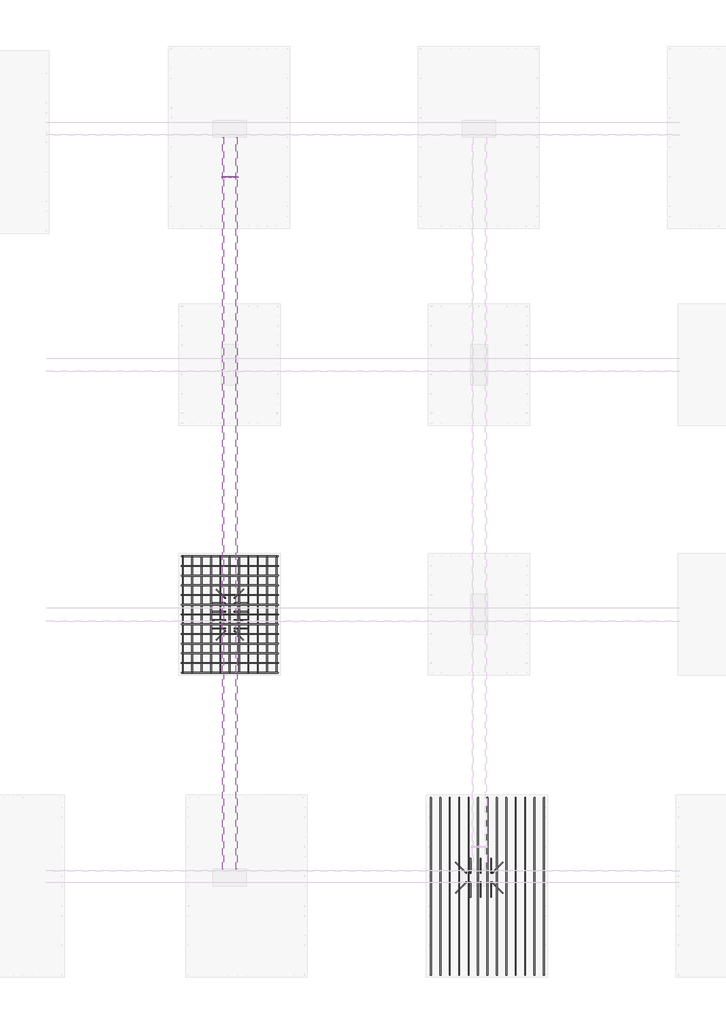
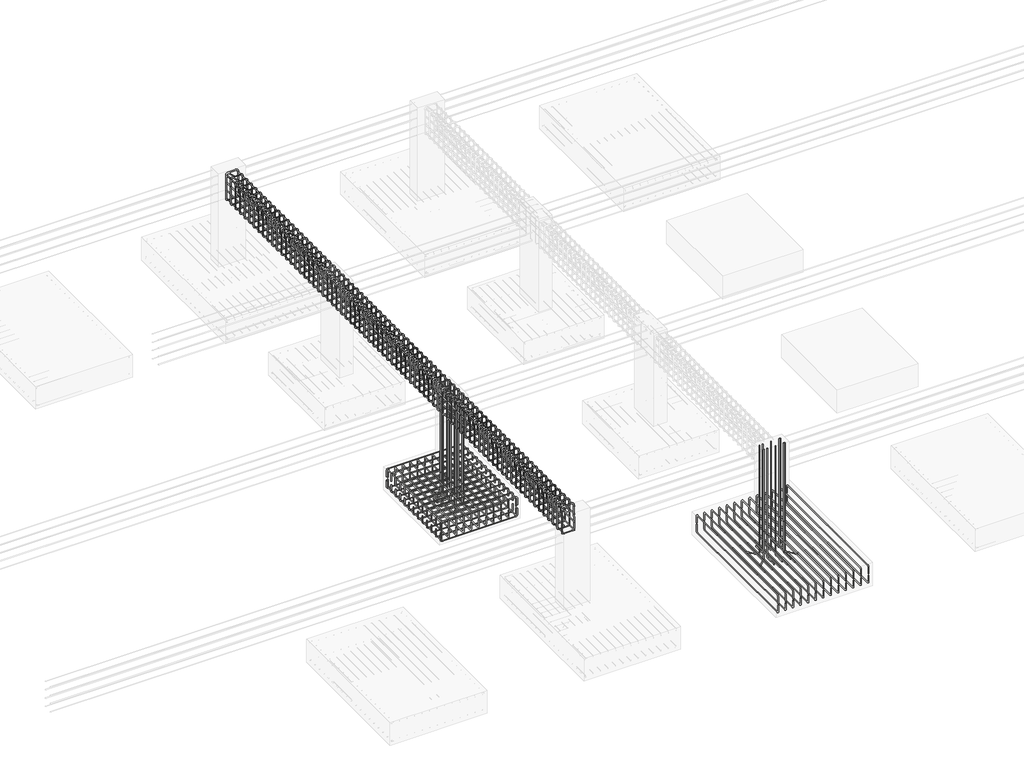
# One storey, part 5 of 16: 21 reinforcing bars.
"""IFC4 building model written with IfcOpenShell, lengths in millimetres."""

from ifc_helpers import new_model, si_unit, point, frame, origin, place, context, project, spatial, polyline, circle_curve, trimmed, segment, composite_curve, source, transform, mapped, element, save
from ifc_brep_helpers import swept_disk

model = new_model("IFC4")

# Units and contexts
model_context = context("Model", 3, world=origin())
ifc_project = project(units=[si_unit("LENGTHUNIT", "METRE", prefix="MILLI")], contexts=[model_context])

# Site, building, storey
site = spatial("IfcSite", under=ifc_project)
building = spatial("IfcBuilding", under=site)
storey = spatial("IfcBuildingStorey", under=building, Elevation=-1828.8)

# Reinforcing bars
placement = place(None, origin())
reinforcing_bar_shape = source(origin(), model_context, "Body", "SolidModel", [
    swept_disk(composite_curve([segment(polyline([(-2445.6525168, -5094.4085501, -2074.8303715), (-2445.6525168, -5094.4085501, -2198.8303715)]), True, "CONTINUOUS"), segment(trimmed(circle_curve(frame((-2445.6525168, -5124.4085501, -2198.8303715), z_axis=(-1.0, 0.0, 0.0), x_axis=(0.0, 30.0, 0.0)), 30.0), [point((-2445.6525168, -5094.4085501, -2198.8303715))], [point((-2445.6525168, -5124.4085501, -2228.8303715))], True, "CARTESIAN"), True, "CONTINUOUS"), segment(polyline([(-2445.6525168, -5124.4085501, -2228.8303715), (-2445.6525168, -7692.4085501, -2228.8303715)]), True, "CONTINUOUS"), segment(trimmed(circle_curve(frame((-2445.6525168, -7692.4085501, -2198.8303715), z_axis=(-1.0, 0.0, 0.0), x_axis=(0.0, 0.0, -30.0)), 30.0), [point((-2445.6525168, -7692.4085501, -2228.8303715))], [point((-2445.6525168, -7722.4085501, -2198.8303715))], True, "CARTESIAN"), True, "CONTINUOUS"), segment(polyline([(-2445.6525168, -7722.4085501, -2198.8303715), (-2445.6525168, -7722.4085501, -2074.8303715)]), True, "CONTINUOUS")], self_intersect=False), 6.0),
])
element("IfcReinforcingBar", 1, at=placement, inside=storey, context=model_context, shape_type="MappedRepresentation", body=[
    mapped(reinforcing_bar_shape, transform((0.0, 0.0, 0.0), x_axis=(1.0, 0.0, 0.0), y_axis=(0.0, 1.0, 0.0), z_axis=(0.0, 0.0, 1.0))),
    mapped(reinforcing_bar_shape, transform((139.7704391, 0.0, 0.0), x_axis=(1.0, 0.0, 0.0), y_axis=(0.0, 1.0, 0.0), z_axis=(0.0, 0.0, 1.0))),
    mapped(reinforcing_bar_shape, transform((279.5408781, 0.0, 0.0), x_axis=(1.0, 0.0, 0.0), y_axis=(0.0, 1.0, 0.0), z_axis=(0.0, 0.0, 1.0))),
    mapped(reinforcing_bar_shape, transform((419.3113172, 0.0, 0.0), x_axis=(1.0, 0.0, 0.0), y_axis=(0.0, 1.0, 0.0), z_axis=(0.0, 0.0, 1.0))),
    mapped(reinforcing_bar_shape, transform((559.0817562, 0.0, 0.0), x_axis=(1.0, 0.0, 0.0), y_axis=(0.0, 1.0, 0.0), z_axis=(0.0, 0.0, 1.0))),
    mapped(reinforcing_bar_shape, transform((698.8521953, 0.0, 0.0), x_axis=(1.0, 0.0, 0.0), y_axis=(0.0, 1.0, 0.0), z_axis=(0.0, 0.0, 1.0))),
    mapped(reinforcing_bar_shape, transform((838.6226343, 0.0, 0.0), x_axis=(1.0, 0.0, 0.0), y_axis=(0.0, 1.0, 0.0), z_axis=(0.0, 0.0, 1.0))),
    mapped(reinforcing_bar_shape, transform((978.3930734, 0.0, 0.0), x_axis=(1.0, 0.0, 0.0), y_axis=(0.0, 1.0, 0.0), z_axis=(0.0, 0.0, 1.0))),
    mapped(reinforcing_bar_shape, transform((1118.1635125, 0.0, 0.0), x_axis=(1.0, 0.0, 0.0), y_axis=(0.0, 1.0, 0.0), z_axis=(0.0, 0.0, 1.0))),
    mapped(reinforcing_bar_shape, transform((1257.9339515, 0.0, 0.0), x_axis=(1.0, 0.0, 0.0), y_axis=(0.0, 1.0, 0.0), z_axis=(0.0, 0.0, 1.0))),
    mapped(reinforcing_bar_shape, transform((1397.7043906, 0.0, 0.0), x_axis=(1.0, 0.0, 0.0), y_axis=(0.0, 1.0, 0.0), z_axis=(0.0, 0.0, 1.0))),
    mapped(reinforcing_bar_shape, transform((1537.4748296, 0.0, 0.0), x_axis=(1.0, 0.0, 0.0), y_axis=(0.0, 1.0, 0.0), z_axis=(0.0, 0.0, 1.0))),
    mapped(reinforcing_bar_shape, transform((1677.2452687, 0.0, 0.0), x_axis=(1.0, 0.0, 0.0), y_axis=(0.0, 1.0, 0.0), z_axis=(0.0, 0.0, 1.0))),
])
reinforcing_bar_2_shape = source(origin(), model_context, "Body", "SolidModel", [
    swept_disk(composite_curve([segment(polyline([(-768.4072481, -5094.4085501, -2038.9453456), (-768.4072481, -5094.4085501, -1914.9453456)]), True, "CONTINUOUS"), segment(trimmed(circle_curve(frame((-768.4072481, -5124.4085501, -1914.9453456), z_axis=(1.0, 0.0, 0.0), x_axis=(0.0, 30.0, 0.0)), 30.0), [point((-768.4072481, -5094.4085501, -1914.9453456))], [point((-768.4072481, -5124.4085501, -1884.9453456))], True, "CARTESIAN"), True, "CONTINUOUS"), segment(polyline([(-768.4072481, -5124.4085501, -1884.9453456), (-768.4072481, -7692.4085501, -1884.9453456)]), True, "CONTINUOUS"), segment(trimmed(circle_curve(frame((-768.4072481, -7692.4085501, -1914.9453456), z_axis=(1.0, 0.0, 0.0), x_axis=(0.0, 0.0, 30.0)), 30.0), [point((-768.4072481, -7692.4085501, -1884.9453456))], [point((-768.4072481, -7722.4085501, -1914.9453456))], True, "CARTESIAN"), True, "CONTINUOUS"), segment(polyline([(-768.4072481, -7722.4085501, -1914.9453456), (-768.4072481, -7722.4085501, -2038.9453456)]), True, "CONTINUOUS")], self_intersect=False), 6.0),
])
element("IfcReinforcingBar", 2, at=placement, inside=storey, context=model_context, shape_type="MappedRepresentation", body=[
    mapped(reinforcing_bar_2_shape, transform((0.0, 0.0, 0.0), x_axis=(1.0, 0.0, 0.0), y_axis=(0.0, 1.0, 0.0), z_axis=(0.0, 0.0, 1.0))),
    mapped(reinforcing_bar_2_shape, transform((-139.7704391, 0.0, 0.0), x_axis=(1.0, 0.0, 0.0), y_axis=(0.0, 1.0, 0.0), z_axis=(0.0, 0.0, 1.0))),
    mapped(reinforcing_bar_2_shape, transform((-279.5408781, 0.0, 0.0), x_axis=(1.0, 0.0, 0.0), y_axis=(0.0, 1.0, 0.0), z_axis=(0.0, 0.0, 1.0))),
    mapped(reinforcing_bar_2_shape, transform((-419.3113172, 0.0, 0.0), x_axis=(1.0, 0.0, 0.0), y_axis=(0.0, 1.0, 0.0), z_axis=(0.0, 0.0, 1.0))),
    mapped(reinforcing_bar_2_shape, transform((-559.0817562, 0.0, 0.0), x_axis=(1.0, 0.0, 0.0), y_axis=(0.0, 1.0, 0.0), z_axis=(0.0, 0.0, 1.0))),
    mapped(reinforcing_bar_2_shape, transform((-698.8521953, 0.0, 0.0), x_axis=(1.0, 0.0, 0.0), y_axis=(0.0, 1.0, 0.0), z_axis=(0.0, 0.0, 1.0))),
    mapped(reinforcing_bar_2_shape, transform((-838.6226343, 0.0, 0.0), x_axis=(1.0, 0.0, 0.0), y_axis=(0.0, 1.0, 0.0), z_axis=(0.0, 0.0, 1.0))),
    mapped(reinforcing_bar_2_shape, transform((-978.3930734, 0.0, 0.0), x_axis=(1.0, 0.0, 0.0), y_axis=(0.0, 1.0, 0.0), z_axis=(0.0, 0.0, 1.0))),
    mapped(reinforcing_bar_2_shape, transform((-1118.1635125, 0.0, 0.0), x_axis=(1.0, 0.0, 0.0), y_axis=(0.0, 1.0, 0.0), z_axis=(0.0, 0.0, 1.0))),
    mapped(reinforcing_bar_2_shape, transform((-1257.9339515, 0.0, 0.0), x_axis=(1.0, 0.0, 0.0), y_axis=(0.0, 1.0, 0.0), z_axis=(0.0, 0.0, 1.0))),
    mapped(reinforcing_bar_2_shape, transform((-1397.7043906, 0.0, 0.0), x_axis=(1.0, 0.0, 0.0), y_axis=(0.0, 1.0, 0.0), z_axis=(0.0, 0.0, 1.0))),
    mapped(reinforcing_bar_2_shape, transform((-1537.4748296, 0.0, 0.0), x_axis=(1.0, 0.0, 0.0), y_axis=(0.0, 1.0, 0.0), z_axis=(0.0, 0.0, 1.0))),
    mapped(reinforcing_bar_2_shape, transform((-1677.2452687, 0.0, 0.0), x_axis=(1.0, 0.0, 0.0), y_axis=(0.0, 1.0, 0.0), z_axis=(0.0, 0.0, 1.0))),
])
reinforcing_bar_3_shape = source(origin(), model_context, "Body", "SolidModel", [
    swept_disk(composite_curve([segment(polyline([(-4714.2725801, -1513.6888221, -2088.8), (-4714.2725801, -1513.6888221, -2212.8)]), True, "CONTINUOUS"), segment(trimmed(circle_curve(frame((-4744.2725801, -1513.6888221, -2212.8), z_axis=(0.0, 1.0, 0.0), x_axis=(30.0, 0.0, 0.0)), 30.0), [point((-4714.2725801, -1513.6888221, -2212.8))], [point((-4744.2725801, -1513.6888221, -2242.8))], True, "CARTESIAN"), True, "CONTINUOUS"), segment(polyline([(-4744.2725801, -1513.6888221, -2242.8), (-6112.2725801, -1513.6888221, -2242.8)]), True, "CONTINUOUS"), segment(trimmed(circle_curve(frame((-6112.2725801, -1513.6888221, -2212.8), z_axis=(0.0, 1.0, 0.0), x_axis=(0.0, 0.0, -30.0)), 30.0), [point((-6112.2725801, -1513.6888221, -2242.8))], [point((-6142.2725801, -1513.6888221, -2212.8))], True, "CARTESIAN"), True, "CONTINUOUS"), segment(polyline([(-6142.2725801, -1513.6888221, -2212.8), (-6142.2725801, -1513.6888221, -2088.8)]), True, "CONTINUOUS")], self_intersect=False), 6.0),
])
element("IfcReinforcingBar", 3, at=placement, inside=storey, context=model_context, shape_type="MappedRepresentation", body=[
    mapped(reinforcing_bar_3_shape, transform((0.0, 0.0, 0.0), x_axis=(1.0, 0.0, 0.0), y_axis=(0.0, 1.0, 0.0), z_axis=(0.0, 0.0, 1.0))),
    mapped(reinforcing_bar_3_shape, transform((0.0, -144.0, 0.0), x_axis=(1.0, 0.0, 0.0), y_axis=(0.0, 1.0, 0.0), z_axis=(0.0, 0.0, 1.0))),
    mapped(reinforcing_bar_3_shape, transform((0.0, -288.0, 0.0), x_axis=(1.0, 0.0, 0.0), y_axis=(0.0, 1.0, 0.0), z_axis=(0.0, 0.0, 1.0))),
    mapped(reinforcing_bar_3_shape, transform((0.0, -432.0, 0.0), x_axis=(1.0, 0.0, 0.0), y_axis=(0.0, 1.0, 0.0), z_axis=(0.0, 0.0, 1.0))),
    mapped(reinforcing_bar_3_shape, transform((0.0, -576.0, 0.0), x_axis=(1.0, 0.0, 0.0), y_axis=(0.0, 1.0, 0.0), z_axis=(0.0, 0.0, 1.0))),
    mapped(reinforcing_bar_3_shape, transform((0.0, -720.0, 0.0), x_axis=(1.0, 0.0, 0.0), y_axis=(0.0, 1.0, 0.0), z_axis=(0.0, 0.0, 1.0))),
    mapped(reinforcing_bar_3_shape, transform((0.0, -864.0, 0.0), x_axis=(1.0, 0.0, 0.0), y_axis=(0.0, 1.0, 0.0), z_axis=(0.0, 0.0, 1.0))),
    mapped(reinforcing_bar_3_shape, transform((0.0, -1008.0, 0.0), x_axis=(1.0, 0.0, 0.0), y_axis=(0.0, 1.0, 0.0), z_axis=(0.0, 0.0, 1.0))),
    mapped(reinforcing_bar_3_shape, transform((0.0, -1152.0, 0.0), x_axis=(1.0, 0.0, 0.0), y_axis=(0.0, 1.0, 0.0), z_axis=(0.0, 0.0, 1.0))),
    mapped(reinforcing_bar_3_shape, transform((0.0, -1296.0, 0.0), x_axis=(1.0, 0.0, 0.0), y_axis=(0.0, 1.0, 0.0), z_axis=(0.0, 0.0, 1.0))),
    mapped(reinforcing_bar_3_shape, transform((0.0, -1440.0, 0.0), x_axis=(1.0, 0.0, 0.0), y_axis=(0.0, 1.0, 0.0), z_axis=(0.0, 0.0, 1.0))),
    mapped(reinforcing_bar_3_shape, transform((0.0, -1584.0, 0.0), x_axis=(1.0, 0.0, 0.0), y_axis=(0.0, 1.0, 0.0), z_axis=(0.0, 0.0, 1.0))),
    mapped(reinforcing_bar_3_shape, transform((0.0, -1728.0, 0.0), x_axis=(1.0, 0.0, 0.0), y_axis=(0.0, 1.0, 0.0), z_axis=(0.0, 0.0, 1.0))),
])
reinforcing_bar_4_shape = source(origin(), model_context, "Body", "SolidModel", [
    swept_disk(composite_curve([segment(polyline([(-6142.2725801, -1513.6888221, -2018.8), (-6142.2725801, -1513.6888221, -1894.8)]), True, "CONTINUOUS"), segment(trimmed(circle_curve(frame((-6112.2725801, -1513.6888221, -1894.8), z_axis=(0.0, 1.0, 0.0), x_axis=(-30.0, 0.0, 0.0)), 30.0), [point((-6142.2725801, -1513.6888221, -1894.8))], [point((-6112.2725801, -1513.6888221, -1864.8))], True, "CARTESIAN"), True, "CONTINUOUS"), segment(polyline([(-6112.2725801, -1513.6888221, -1864.8), (-4744.2725801, -1513.6888221, -1864.8)]), True, "CONTINUOUS"), segment(trimmed(circle_curve(frame((-4744.2725801, -1513.6888221, -1894.8), z_axis=(0.0, 1.0, 0.0), x_axis=(0.0, 0.0, 30.0)), 30.0), [point((-4744.2725801, -1513.6888221, -1864.8))], [point((-4714.2725801, -1513.6888221, -1894.8))], True, "CARTESIAN"), True, "CONTINUOUS"), segment(polyline([(-4714.2725801, -1513.6888221, -1894.8), (-4714.2725801, -1513.6888221, -2018.8)]), True, "CONTINUOUS")], self_intersect=False), 6.0),
])
element("IfcReinforcingBar", 4, at=placement, inside=storey, context=model_context, shape_type="MappedRepresentation", body=[
    mapped(reinforcing_bar_4_shape, transform((0.0, 0.0, 0.0), x_axis=(1.0, 0.0, 0.0), y_axis=(0.0, 1.0, 0.0), z_axis=(0.0, 0.0, 1.0))),
    mapped(reinforcing_bar_4_shape, transform((0.0, -144.0, 0.0), x_axis=(1.0, 0.0, 0.0), y_axis=(0.0, 1.0, 0.0), z_axis=(0.0, 0.0, 1.0))),
    mapped(reinforcing_bar_4_shape, transform((0.0, -288.0, 0.0), x_axis=(1.0, 0.0, 0.0), y_axis=(0.0, 1.0, 0.0), z_axis=(0.0, 0.0, 1.0))),
    mapped(reinforcing_bar_4_shape, transform((0.0, -432.0, 0.0), x_axis=(1.0, 0.0, 0.0), y_axis=(0.0, 1.0, 0.0), z_axis=(0.0, 0.0, 1.0))),
    mapped(reinforcing_bar_4_shape, transform((0.0, -576.0, 0.0), x_axis=(1.0, 0.0, 0.0), y_axis=(0.0, 1.0, 0.0), z_axis=(0.0, 0.0, 1.0))),
    mapped(reinforcing_bar_4_shape, transform((0.0, -720.0, 0.0), x_axis=(1.0, 0.0, 0.0), y_axis=(0.0, 1.0, 0.0), z_axis=(0.0, 0.0, 1.0))),
    mapped(reinforcing_bar_4_shape, transform((0.0, -864.0, 0.0), x_axis=(1.0, 0.0, 0.0), y_axis=(0.0, 1.0, 0.0), z_axis=(0.0, 0.0, 1.0))),
    mapped(reinforcing_bar_4_shape, transform((0.0, -1008.0, 0.0), x_axis=(1.0, 0.0, 0.0), y_axis=(0.0, 1.0, 0.0), z_axis=(0.0, 0.0, 1.0))),
    mapped(reinforcing_bar_4_shape, transform((0.0, -1152.0, 0.0), x_axis=(1.0, 0.0, 0.0), y_axis=(0.0, 1.0, 0.0), z_axis=(0.0, 0.0, 1.0))),
    mapped(reinforcing_bar_4_shape, transform((0.0, -1296.0, 0.0), x_axis=(1.0, 0.0, 0.0), y_axis=(0.0, 1.0, 0.0), z_axis=(0.0, 0.0, 1.0))),
    mapped(reinforcing_bar_4_shape, transform((0.0, -1440.0, 0.0), x_axis=(1.0, 0.0, 0.0), y_axis=(0.0, 1.0, 0.0), z_axis=(0.0, 0.0, 1.0))),
    mapped(reinforcing_bar_4_shape, transform((0.0, -1584.0, 0.0), x_axis=(1.0, 0.0, 0.0), y_axis=(0.0, 1.0, 0.0), z_axis=(0.0, 0.0, 1.0))),
    mapped(reinforcing_bar_4_shape, transform((0.0, -1728.0, 0.0), x_axis=(1.0, 0.0, 0.0), y_axis=(0.0, 1.0, 0.0), z_axis=(0.0, 0.0, 1.0))),
])
reinforcing_bar_5_shape = source(origin(), model_context, "Body", "SolidModel", [
    swept_disk(composite_curve([segment(polyline([(-6125.0397909, -1513.6888221, -2072.0951729), (-6125.0397909, -1513.6888221, -2196.0951729)]), True, "CONTINUOUS"), segment(trimmed(circle_curve(frame((-6125.0397909, -1543.6888221, -2196.0951729), z_axis=(-1.0, 0.0, 0.0), x_axis=(0.0, 30.0, 0.0)), 30.0), [point((-6125.0397909, -1513.6888221, -2196.0951729))], [point((-6125.0397909, -1543.6888221, -2226.0951729))], True, "CARTESIAN"), True, "CONTINUOUS"), segment(polyline([(-6125.0397909, -1543.6888221, -2226.0951729), (-6125.0397909, -3211.6888221, -2226.0951729)]), True, "CONTINUOUS"), segment(trimmed(circle_curve(frame((-6125.0397909, -3211.6888221, -2196.0951729), z_axis=(-1.0, 0.0, 0.0), x_axis=(0.0, 0.0, -30.0)), 30.0), [point((-6125.0397909, -3211.6888221, -2226.0951729))], [point((-6125.0397909, -3241.6888221, -2196.0951729))], True, "CARTESIAN"), True, "CONTINUOUS"), segment(polyline([(-6125.0397909, -3241.6888221, -2196.0951729), (-6125.0397909, -3241.6888221, -2072.0951729)]), True, "CONTINUOUS")], self_intersect=False), 6.0),
])
element("IfcReinforcingBar", 5, at=placement, inside=storey, context=model_context, shape_type="MappedRepresentation", body=[
    mapped(reinforcing_bar_5_shape, transform((0.0, 0.0, 0.0), x_axis=(1.0, 0.0, 0.0), y_axis=(0.0, 1.0, 0.0), z_axis=(0.0, 0.0, 1.0))),
    mapped(reinforcing_bar_5_shape, transform((138.8820351, 0.0, 0.0), x_axis=(1.0, 0.0, 0.0), y_axis=(0.0, 1.0, 0.0), z_axis=(0.0, 0.0, 1.0))),
    mapped(reinforcing_bar_5_shape, transform((277.7640703, 0.0, 0.0), x_axis=(1.0, 0.0, 0.0), y_axis=(0.0, 1.0, 0.0), z_axis=(0.0, 0.0, 1.0))),
    mapped(reinforcing_bar_5_shape, transform((416.6461054, 0.0, 0.0), x_axis=(1.0, 0.0, 0.0), y_axis=(0.0, 1.0, 0.0), z_axis=(0.0, 0.0, 1.0))),
    mapped(reinforcing_bar_5_shape, transform((555.5281406, 0.0, 0.0), x_axis=(1.0, 0.0, 0.0), y_axis=(0.0, 1.0, 0.0), z_axis=(0.0, 0.0, 1.0))),
    mapped(reinforcing_bar_5_shape, transform((694.4101757, 0.0, 0.0), x_axis=(1.0, 0.0, 0.0), y_axis=(0.0, 1.0, 0.0), z_axis=(0.0, 0.0, 1.0))),
    mapped(reinforcing_bar_5_shape, transform((833.2922109, 0.0, 0.0), x_axis=(1.0, 0.0, 0.0), y_axis=(0.0, 1.0, 0.0), z_axis=(0.0, 0.0, 1.0))),
    mapped(reinforcing_bar_5_shape, transform((972.174246, 0.0, 0.0), x_axis=(1.0, 0.0, 0.0), y_axis=(0.0, 1.0, 0.0), z_axis=(0.0, 0.0, 1.0))),
    mapped(reinforcing_bar_5_shape, transform((1111.0562811, 0.0, 0.0), x_axis=(1.0, 0.0, 0.0), y_axis=(0.0, 1.0, 0.0), z_axis=(0.0, 0.0, 1.0))),
    mapped(reinforcing_bar_5_shape, transform((1249.9383163, 0.0, 0.0), x_axis=(1.0, 0.0, 0.0), y_axis=(0.0, 1.0, 0.0), z_axis=(0.0, 0.0, 1.0))),
    mapped(reinforcing_bar_5_shape, transform((1388.8203514, 0.0, 0.0), x_axis=(1.0, 0.0, 0.0), y_axis=(0.0, 1.0, 0.0), z_axis=(0.0, 0.0, 1.0))),
])
reinforcing_bar_6_shape = source(origin(), model_context, "Body", "SolidModel", [
    swept_disk(composite_curve([segment(polyline([(-4736.2194394, -1513.6888221, -2034.1277079), (-4736.2194394, -1513.6888221, -1910.1277079)]), True, "CONTINUOUS"), segment(trimmed(circle_curve(frame((-4736.2194394, -1543.6888221, -1910.1277079), z_axis=(1.0, 0.0, 0.0), x_axis=(0.0, 30.0, 0.0)), 30.0), [point((-4736.2194394, -1513.6888221, -1910.1277079))], [point((-4736.2194394, -1543.6888221, -1880.1277079))], True, "CARTESIAN"), True, "CONTINUOUS"), segment(polyline([(-4736.2194394, -1543.6888221, -1880.1277079), (-4736.2194394, -3211.6888221, -1880.1277079)]), True, "CONTINUOUS"), segment(trimmed(circle_curve(frame((-4736.2194394, -3211.6888221, -1910.1277079), z_axis=(1.0, 0.0, 0.0), x_axis=(0.0, 0.0, 30.0)), 30.0), [point((-4736.2194394, -3211.6888221, -1880.1277079))], [point((-4736.2194394, -3241.6888221, -1910.1277079))], True, "CARTESIAN"), True, "CONTINUOUS"), segment(polyline([(-4736.2194394, -3241.6888221, -1910.1277079), (-4736.2194394, -3241.6888221, -2034.1277079)]), True, "CONTINUOUS")], self_intersect=False), 6.0),
])
element("IfcReinforcingBar", 6, at=placement, inside=storey, context=model_context, shape_type="MappedRepresentation", body=[
    mapped(reinforcing_bar_6_shape, transform((0.0, 0.0, 0.0), x_axis=(1.0, 0.0, 0.0), y_axis=(0.0, 1.0, 0.0), z_axis=(0.0, 0.0, 1.0))),
    mapped(reinforcing_bar_6_shape, transform((-138.8820351, 0.0, 0.0), x_axis=(1.0, 0.0, 0.0), y_axis=(0.0, 1.0, 0.0), z_axis=(0.0, 0.0, 1.0))),
    mapped(reinforcing_bar_6_shape, transform((-277.7640703, 0.0, 0.0), x_axis=(1.0, 0.0, 0.0), y_axis=(0.0, 1.0, 0.0), z_axis=(0.0, 0.0, 1.0))),
    mapped(reinforcing_bar_6_shape, transform((-416.6461054, 0.0, 0.0), x_axis=(1.0, 0.0, 0.0), y_axis=(0.0, 1.0, 0.0), z_axis=(0.0, 0.0, 1.0))),
    mapped(reinforcing_bar_6_shape, transform((-555.5281406, 0.0, 0.0), x_axis=(1.0, 0.0, 0.0), y_axis=(0.0, 1.0, 0.0), z_axis=(0.0, 0.0, 1.0))),
    mapped(reinforcing_bar_6_shape, transform((-694.4101757, 0.0, 0.0), x_axis=(1.0, 0.0, 0.0), y_axis=(0.0, 1.0, 0.0), z_axis=(0.0, 0.0, 1.0))),
    mapped(reinforcing_bar_6_shape, transform((-833.2922109, 0.0, 0.0), x_axis=(1.0, 0.0, 0.0), y_axis=(0.0, 1.0, 0.0), z_axis=(0.0, 0.0, 1.0))),
    mapped(reinforcing_bar_6_shape, transform((-972.174246, 0.0, 0.0), x_axis=(1.0, 0.0, 0.0), y_axis=(0.0, 1.0, 0.0), z_axis=(0.0, 0.0, 1.0))),
    mapped(reinforcing_bar_6_shape, transform((-1111.0562811, 0.0, 0.0), x_axis=(1.0, 0.0, 0.0), y_axis=(0.0, 1.0, 0.0), z_axis=(0.0, 0.0, 1.0))),
    mapped(reinforcing_bar_6_shape, transform((-1249.9383163, 0.0, 0.0), x_axis=(1.0, 0.0, 0.0), y_axis=(0.0, 1.0, 0.0), z_axis=(0.0, 0.0, 1.0))),
    mapped(reinforcing_bar_6_shape, transform((-1388.8203514, 0.0, 0.0), x_axis=(1.0, 0.0, 0.0), y_axis=(0.0, 1.0, 0.0), z_axis=(0.0, 0.0, 1.0))),
])
reinforcing_bar_7_shape = source(origin(), model_context, "Body", "SolidModel", [
    swept_disk(composite_curve([segment(polyline([(-1860.102427, -6208.8808991, -30.0), (-1860.102427, -6208.8808991, -2141.7459972)]), True, "CONTINUOUS"), segment(trimmed(circle_curve(frame((-1860.102427, -6178.8808991, -2141.7459972), z_axis=(1.0, 0.0, 0.0), x_axis=(0.0, -30.0, 0.0)), 30.0), [point((-1860.102427, -6208.8808991, -2141.7459972))], [point((-1860.102427, -6178.8808991, -2171.7459972))], True, "CARTESIAN"), True, "CONTINUOUS"), segment(polyline([(-1860.102427, -6178.8808991, -2171.7459972), (-1860.102427, -5988.2528007, -2171.7459972)]), True, "CONTINUOUS")], self_intersect=False), 6.0),
])
element("IfcReinforcingBar", 7, at=placement, inside=storey, context=model_context, shape_type="MappedRepresentation", body=[
    mapped(reinforcing_bar_7_shape, transform((0.0, 0.0, 0.0), x_axis=(1.0, 0.0, 0.0), y_axis=(0.0, 1.0, 0.0), z_axis=(0.0, 0.0, 1.0))),
    mapped(reinforcing_bar_7_shape, transform((153.9273626, 0.0, 0.0), x_axis=(1.0, 0.0, 0.0), y_axis=(0.0, 1.0, 0.0), z_axis=(0.0, 0.0, 1.0))),
    mapped(reinforcing_bar_7_shape, transform((307.8547253, 0.0, 0.0), x_axis=(1.0, 0.0, 0.0), y_axis=(0.0, 1.0, 0.0), z_axis=(0.0, 0.0, 1.0))),
])
element("IfcReinforcingBar", 8, at=placement, inside=storey, context=model_context, shape_type="SolidModel", body=[
    swept_disk(composite_curve([segment(polyline([(-1921.7720578, -6208.8808991, -30.0), (-1921.7720578, -6208.8808991, -2141.7459972)]), True, "CONTINUOUS"), segment(trimmed(circle_curve(frame((-1942.9852612, -6187.6676957, -2141.7459972), z_axis=(0.7071067811865476, 0.7071067811865475, 0.0), x_axis=(21.213203399999884, -21.213203399999657, 0.0)), 30.0), [point((-1921.7720578, -6208.8808991, -2141.7459972))], [point((-1942.9852612, -6187.6676957, -2171.7459972))], True, "CARTESIAN"), True, "CONTINUOUS"), segment(polyline([(-1942.9852612, -6187.6676957, -2171.7459972), (-2077.7796823, -6052.8732746, -2171.7459972)]), True, "CONTINUOUS")], self_intersect=False), 6.0),
])
element("IfcReinforcingBar", 9, at=placement, inside=storey, context=model_context, shape_type="SolidModel", body=[
    swept_disk(composite_curve([segment(polyline([(-1921.7720578, -6349.3808991, -30.0), (-1921.7720578, -6349.3808991, -2141.7459972)]), True, "CONTINUOUS"), segment(trimmed(circle_curve(frame((-1942.9852612, -6370.5941026, -2141.7459972), z_axis=(-0.7071067811865444, 0.7071067811865507, 0.0), x_axis=(21.213203399999884, 21.213203500000418, 0.0)), 30.0), [point((-1921.7720578, -6349.3808991, -2141.7459972))], [point((-1942.9852612, -6370.5941026, -2171.7459972))], True, "CARTESIAN"), True, "CONTINUOUS"), segment(polyline([(-1942.9852612, -6370.5941026, -2171.7459972), (-2077.7796823, -6505.3885237, -2171.7459972)]), True, "CONTINUOUS")], self_intersect=False), 6.0),
])
element("IfcReinforcingBar", 10, at=placement, inside=storey, context=model_context, shape_type="SolidModel", body=[
    swept_disk(composite_curve([segment(polyline([(-1534.7731024, -6349.3808991, -30.0), (-1534.7731024, -6349.3808991, -2141.7459972)]), True, "CONTINUOUS"), segment(trimmed(circle_curve(frame((-1513.559899, -6370.5941026, -2141.7459972), z_axis=(-0.7071067811865445, -0.7071067811865506, 0.0), x_axis=(-21.213203399999884, 21.213203500000418, 0.0)), 30.0), [point((-1534.7731024, -6349.3808991, -2141.7459972))], [point((-1513.559899, -6370.5941026, -2171.7459972))], True, "CARTESIAN"), True, "CONTINUOUS"), segment(polyline([(-1513.559899, -6370.5941026, -2171.7459972), (-1378.7654779, -6505.3885237, -2171.7459972)]), True, "CONTINUOUS")], self_intersect=False), 6.0),
])
element("IfcReinforcingBar", 11, at=placement, inside=storey, context=model_context, shape_type="SolidModel", body=[
    swept_disk(composite_curve([segment(polyline([(-1534.7731024, -6208.8808991, -30.0), (-1534.7731024, -6208.8808991, -2141.7459972)]), True, "CONTINUOUS"), segment(trimmed(circle_curve(frame((-1513.559899, -6187.6676957, -2141.7459972), z_axis=(0.7071067811865476, -0.7071067811865476, 0.0), x_axis=(-21.213203399999884, -21.213203399999657, 0.0)), 30.0), [point((-1534.7731024, -6208.8808991, -2141.7459972))], [point((-1513.559899, -6187.6676957, -2171.7459972))], True, "CARTESIAN"), True, "CONTINUOUS"), segment(polyline([(-1513.559899, -6187.6676957, -2171.7459972), (-1378.7654779, -6052.8732746, -2171.7459972)]), True, "CONTINUOUS")], self_intersect=False), 6.0),
])
reinforcing_bar_8_shape = source(origin(), model_context, "Body", "SolidModel", [
    swept_disk(composite_curve([segment(polyline([(-1860.102427, -6349.3808991, -30.0), (-1860.102427, -6349.3808991, -2141.7459972)]), True, "CONTINUOUS"), segment(trimmed(circle_curve(frame((-1860.102427, -6379.3808991, -2141.7459972), z_axis=(-1.0, 0.0, 0.0), x_axis=(0.0, 30.0, 0.0)), 30.0), [point((-1860.102427, -6349.3808991, -2141.7459972))], [point((-1860.102427, -6379.3808991, -2171.7459972))], True, "CARTESIAN"), True, "CONTINUOUS"), segment(polyline([(-1860.102427, -6379.3808991, -2171.7459972), (-1860.102427, -6570.0089976, -2171.7459972)]), True, "CONTINUOUS")], self_intersect=False), 6.0),
])
element("IfcReinforcingBar", 12, at=placement, inside=storey, context=model_context, shape_type="MappedRepresentation", body=[
    mapped(reinforcing_bar_8_shape, transform((0.0, 0.0, 0.0), x_axis=(1.0, 0.0, 0.0), y_axis=(0.0, 1.0, 0.0), z_axis=(0.0, 0.0, 1.0))),
    mapped(reinforcing_bar_8_shape, transform((153.9273626, 0.0, 0.0), x_axis=(1.0, 0.0, 0.0), y_axis=(0.0, 1.0, 0.0), z_axis=(0.0, 0.0, 1.0))),
    mapped(reinforcing_bar_8_shape, transform((307.8547253, 0.0, 0.0), x_axis=(1.0, 0.0, 0.0), y_axis=(0.0, 1.0, 0.0), z_axis=(0.0, 0.0, 1.0))),
])
reinforcing_bar_9_shape = source(origin(), model_context, "Body", "SolidModel", [
    swept_disk(composite_curve([segment(polyline([(-5358.2317051, -2212.2776925, -30.0), (-5358.2317051, -2212.2776925, -2158.8)]), True, "CONTINUOUS"), segment(trimmed(circle_curve(frame((-5328.2317051, -2212.2776925, -2158.8), z_axis=(0.0, -1.0, 0.0), x_axis=(-30.0, 0.0, 0.0)), 30.0), [point((-5358.2317051, -2212.2776925, -2158.8))], [point((-5328.2317051, -2212.2776925, -2188.8))], True, "CARTESIAN"), True, "CONTINUOUS"), segment(polyline([(-5328.2317051, -2212.2776925, -2188.8), (-5175.8458602, -2212.2776925, -2188.8)]), True, "CONTINUOUS")], self_intersect=False), 6.0),
])
element("IfcReinforcingBar", 13, at=placement, inside=storey, context=model_context, shape_type="MappedRepresentation", body=[
    mapped(reinforcing_bar_9_shape, transform((0.0, 0.0, 0.0), x_axis=(1.0, 0.0, 0.0), y_axis=(0.0, 1.0, 0.0), z_axis=(0.0, 0.0, 1.0))),
    mapped(reinforcing_bar_9_shape, transform((0.0, -123.8384715, 0.0), x_axis=(1.0, 0.0, 0.0), y_axis=(0.0, 1.0, 0.0), z_axis=(0.0, 0.0, 1.0))),
    mapped(reinforcing_bar_9_shape, transform((0.0, -247.676943, 0.0), x_axis=(1.0, 0.0, 0.0), y_axis=(0.0, 1.0, 0.0), z_axis=(0.0, 0.0, 1.0))),
    mapped(reinforcing_bar_9_shape, transform((0.0, -371.5154145, 0.0), x_axis=(1.0, 0.0, 0.0), y_axis=(0.0, 1.0, 0.0), z_axis=(0.0, 0.0, 1.0))),
])
element("IfcReinforcingBar", 14, at=placement, inside=storey, context=model_context, shape_type="SolidModel", body=[
    swept_disk(composite_curve([segment(polyline([(-5498.3134551, -2134.0900242, -30.0), (-5498.3134551, -2134.0900242, -2158.8)]), True, "CONTINUOUS"), segment(trimmed(circle_curve(frame((-5519.5266585, -2112.8768207, -2158.8), z_axis=(0.7071067811865435, 0.7071067811865517, 0.0), x_axis=(21.213203399999657, -21.213203499999963, 0.0)), 30.0), [point((-5498.3134551, -2134.0900242, -2158.8))], [point((-5519.5266585, -2112.8768207, -2188.8))], True, "CARTESIAN"), True, "CONTINUOUS"), segment(polyline([(-5519.5266585, -2112.8768207, -2188.8), (-5627.2797228, -2005.1237565, -2188.8)]), True, "CONTINUOUS")], self_intersect=False), 6.0),
])
element("IfcReinforcingBar", 15, at=placement, inside=storey, context=model_context, shape_type="SolidModel", body=[
    swept_disk(composite_curve([segment(polyline([(-5358.2317051, -2624.1717741, -30.0), (-5358.2317051, -2624.1717741, -2158.8)]), True, "CONTINUOUS"), segment(trimmed(circle_curve(frame((-5337.0185017, -2645.3849776, -2158.8), z_axis=(-0.7071067811865435, -0.7071067811865516, 0.0), x_axis=(-21.213203399999657, 21.213203499999963, 0.0)), 30.0), [point((-5358.2317051, -2624.1717741, -2158.8))], [point((-5337.0185017, -2645.3849776, -2188.8))], True, "CARTESIAN"), True, "CONTINUOUS"), segment(polyline([(-5337.0185017, -2645.3849776, -2188.8), (-5229.2654374, -2753.1380418, -2188.8)]), True, "CONTINUOUS")], self_intersect=False), 6.0),
])
element("IfcReinforcingBar", 16, at=placement, inside=storey, context=model_context, shape_type="SolidModel", body=[
    swept_disk(composite_curve([segment(polyline([(-5498.3134551, -2624.1717741, -30.0), (-5498.3134551, -2624.1717741, -2158.8)]), True, "CONTINUOUS"), segment(trimmed(circle_curve(frame((-5519.5266585, -2645.3849776, -2158.8), z_axis=(-0.7071067811865436, 0.7071067811865517, 0.0), x_axis=(21.213203399999657, 21.213203499999963, 0.0)), 30.0), [point((-5498.3134551, -2624.1717741, -2158.8))], [point((-5519.5266585, -2645.3849776, -2188.8))], True, "CARTESIAN"), True, "CONTINUOUS"), segment(polyline([(-5519.5266585, -2645.3849776, -2188.8), (-5627.2797228, -2753.1380418, -2188.8)]), True, "CONTINUOUS")], self_intersect=False), 6.0),
])
element("IfcReinforcingBar", 17, at=placement, inside=storey, context=model_context, shape_type="SolidModel", body=[
    swept_disk(composite_curve([segment(polyline([(-5358.2317051, -2134.0900242, -30.0), (-5358.2317051, -2134.0900242, -2158.8)]), True, "CONTINUOUS"), segment(trimmed(circle_curve(frame((-5337.0185017, -2112.8768207, -2158.8), z_axis=(0.7071067811865436, -0.7071067811865517, 0.0), x_axis=(-21.213203399999657, -21.213203499999963, 0.0)), 30.0), [point((-5358.2317051, -2134.0900242, -2158.8))], [point((-5337.0185017, -2112.8768207, -2188.8))], True, "CARTESIAN"), True, "CONTINUOUS"), segment(polyline([(-5337.0185017, -2112.8768207, -2188.8), (-5229.2654374, -2005.1237565, -2188.8)]), True, "CONTINUOUS")], self_intersect=False), 6.0),
])
reinforcing_bar_10_shape = source(origin(), model_context, "Body", "SolidModel", [
    swept_disk(composite_curve([segment(polyline([(-5498.3134551, -2212.2776925, -30.0), (-5498.3134551, -2212.2776925, -2158.8)]), True, "CONTINUOUS"), segment(trimmed(circle_curve(frame((-5528.3134551, -2212.2776925, -2158.8), z_axis=(0.0, 1.0, 0.0), x_axis=(30.0, 0.0, 0.0)), 30.0), [point((-5498.3134551, -2212.2776925, -2158.8))], [point((-5528.3134551, -2212.2776925, -2188.8))], True, "CARTESIAN"), True, "CONTINUOUS"), segment(polyline([(-5528.3134551, -2212.2776925, -2188.8), (-5680.6992999, -2212.2776925, -2188.8)]), True, "CONTINUOUS")], self_intersect=False), 6.0),
])
element("IfcReinforcingBar", 18, at=placement, inside=storey, context=model_context, shape_type="MappedRepresentation", body=[
    mapped(reinforcing_bar_10_shape, transform((0.0, 0.0, 0.0), x_axis=(1.0, 0.0, 0.0), y_axis=(0.0, 1.0, 0.0), z_axis=(0.0, 0.0, 1.0))),
    mapped(reinforcing_bar_10_shape, transform((0.0, -123.8384715, 0.0), x_axis=(1.0, 0.0, 0.0), y_axis=(0.0, 1.0, 0.0), z_axis=(0.0, 0.0, 1.0))),
    mapped(reinforcing_bar_10_shape, transform((0.0, -247.676943, 0.0), x_axis=(1.0, 0.0, 0.0), y_axis=(0.0, 1.0, 0.0), z_axis=(0.0, 0.0, 1.0))),
    mapped(reinforcing_bar_10_shape, transform((0.0, -371.5154145, 0.0), x_axis=(1.0, 0.0, 0.0), y_axis=(0.0, 1.0, 0.0), z_axis=(0.0, 0.0, 1.0))),
])
reinforcing_bar_11_shape = source(origin(), model_context, "Body", "SolidModel", [
    swept_disk(composite_curve([segment(polyline([(-5403.3781358, 4695.8691009, -132.4680374), (-5491.0593767, 4695.8691009, -44.7867966)]), True, "CONTINUOUS"), segment(trimmed(circle_curve(frame((-5512.2725801, 4695.8691009, -66.0), z_axis=(0.0, -1.0, 0.0), x_axis=(21.213203399999657, 0.0, 21.213203399999998)), 30.0), [point((-5491.0593767, 4695.8691009, -44.7867966))], [point((-5542.2725801, 4695.8691009, -66.0))], True, "CARTESIAN"), True, "CONTINUOUS"), segment(polyline([(-5542.2725801, 4695.8691009, -66.0), (-5542.2725801, 4695.8691009, -534.0)]), True, "CONTINUOUS"), segment(trimmed(circle_curve(frame((-5512.2725801, 4695.8691009, -534.0), z_axis=(0.0, -1.0, 0.0), x_axis=(-30.0, 0.0, 0.0)), 30.0), [point((-5542.2725801, 4695.8691009, -534.0))], [point((-5512.2725801, 4695.8691009, -564.0))], True, "CARTESIAN"), True, "CONTINUOUS"), segment(polyline([(-5512.2725801, 4695.8691009, -564.0), (-5344.2725801, 4695.8691009, -564.0)]), True, "CONTINUOUS"), segment(trimmed(circle_curve(frame((-5344.2725801, 4696.550743, -534.0077449), z_axis=(0.0, -0.9997418355449428, 0.022721405353294154), x_axis=(0.0, -0.681642099999408, -29.992255099999966)), 30.0), [point((-5344.2725801, 4695.8691009, -564.0))], [point((-5314.2725801, 4696.550743, -534.0077449))], True, "CARTESIAN"), True, "CONTINUOUS"), segment(polyline([(-5314.2725801, 4696.550743, -534.0077449), (-5314.2725801, 4707.1874587, -65.9922551)]), True, "CONTINUOUS"), segment(trimmed(circle_curve(frame((-5344.2725801, 4707.1874587, -65.9922551), z_axis=(0.0, -0.9997418355449428, 0.022721405353294154), x_axis=(30.0, 0.0, 0.0)), 30.0), [point((-5314.2725801, 4707.1874587, -65.9922551))], [point((-5344.2725801, 4707.8691009, -36.0))], True, "CARTESIAN"), True, "CONTINUOUS"), segment(polyline([(-5344.2725801, 4707.8691009, -36.0), (-5512.2725801, 4707.8691009, -36.0)]), True, "CONTINUOUS"), segment(trimmed(circle_curve(frame((-5512.2725801, 4707.8691009, -66.0), z_axis=(0.0, -1.0, 0.0), x_axis=(0.0, 0.0, 30.0)), 30.0), [point((-5512.2725801, 4707.8691009, -36.0))], [point((-5533.4857835, 4707.8691009, -87.2132034))], True, "CARTESIAN"), True, "CONTINUOUS"), segment(polyline([(-5533.4857835, 4707.8691009, -87.2132034), (-5445.8045427, 4707.8691009, -174.8944443)]), True, "CONTINUOUS")], self_intersect=False), 6.0),
])
element("IfcReinforcingBar", 19, at=placement, inside=storey, context=model_context, shape_type="MappedRepresentation", body=[
    mapped(reinforcing_bar_11_shape, transform((0.0, 0.0, 0.0), x_axis=(1.0, 0.0, 0.0), y_axis=(0.0, 1.0, 0.0), z_axis=(0.0, 0.0, 1.0))),
    mapped(reinforcing_bar_11_shape, transform((0.0, -148.1212116, 0.0), x_axis=(1.0, 0.0, 0.0), y_axis=(0.0, 1.0, 0.0), z_axis=(0.0, 0.0, 1.0))),
    mapped(reinforcing_bar_11_shape, transform((0.0, -296.2424232, 0.0), x_axis=(1.0, 0.0, 0.0), y_axis=(0.0, 1.0, 0.0), z_axis=(0.0, 0.0, 1.0))),
    mapped(reinforcing_bar_11_shape, transform((0.0, -444.3636348, 0.0), x_axis=(1.0, 0.0, 0.0), y_axis=(0.0, 1.0, 0.0), z_axis=(0.0, 0.0, 1.0))),
    mapped(reinforcing_bar_11_shape, transform((0.0, -592.4848465, 0.0), x_axis=(1.0, 0.0, 0.0), y_axis=(0.0, 1.0, 0.0), z_axis=(0.0, 0.0, 1.0))),
    mapped(reinforcing_bar_11_shape, transform((0.0, -740.6060581, 0.0), x_axis=(1.0, 0.0, 0.0), y_axis=(0.0, 1.0, 0.0), z_axis=(0.0, 0.0, 1.0))),
    mapped(reinforcing_bar_11_shape, transform((0.0, -888.7272697, 0.0), x_axis=(1.0, 0.0, 0.0), y_axis=(0.0, 1.0, 0.0), z_axis=(0.0, 0.0, 1.0))),
    mapped(reinforcing_bar_11_shape, transform((0.0, -1036.8484813, 0.0), x_axis=(1.0, 0.0, 0.0), y_axis=(0.0, 1.0, 0.0), z_axis=(0.0, 0.0, 1.0))),
    mapped(reinforcing_bar_11_shape, transform((0.0, -1184.9696929, 0.0), x_axis=(1.0, 0.0, 0.0), y_axis=(0.0, 1.0, 0.0), z_axis=(0.0, 0.0, 1.0))),
    mapped(reinforcing_bar_11_shape, transform((0.0, -1333.0909045, 0.0), x_axis=(1.0, 0.0, 0.0), y_axis=(0.0, 1.0, 0.0), z_axis=(0.0, 0.0, 1.0))),
    mapped(reinforcing_bar_11_shape, transform((0.0, -1481.2121161, 0.0), x_axis=(1.0, 0.0, 0.0), y_axis=(0.0, 1.0, 0.0), z_axis=(0.0, 0.0, 1.0))),
    mapped(reinforcing_bar_11_shape, transform((0.0, -1629.3333278, 0.0), x_axis=(1.0, 0.0, 0.0), y_axis=(0.0, 1.0, 0.0), z_axis=(0.0, 0.0, 1.0))),
    mapped(reinforcing_bar_11_shape, transform((0.0, -1777.4545394, 0.0), x_axis=(1.0, 0.0, 0.0), y_axis=(0.0, 1.0, 0.0), z_axis=(0.0, 0.0, 1.0))),
    mapped(reinforcing_bar_11_shape, transform((0.0, -1925.575751, 0.0), x_axis=(1.0, 0.0, 0.0), y_axis=(0.0, 1.0, 0.0), z_axis=(0.0, 0.0, 1.0))),
    mapped(reinforcing_bar_11_shape, transform((0.0, -2073.6969626, 0.0), x_axis=(1.0, 0.0, 0.0), y_axis=(0.0, 1.0, 0.0), z_axis=(0.0, 0.0, 1.0))),
    mapped(reinforcing_bar_11_shape, transform((0.0, -2221.8181742, 0.0), x_axis=(1.0, 0.0, 0.0), y_axis=(0.0, 1.0, 0.0), z_axis=(0.0, 0.0, 1.0))),
    mapped(reinforcing_bar_11_shape, transform((0.0, -2369.9393858, 0.0), x_axis=(1.0, 0.0, 0.0), y_axis=(0.0, 1.0, 0.0), z_axis=(0.0, 0.0, 1.0))),
    mapped(reinforcing_bar_11_shape, transform((0.0, -2518.0605974, 0.0), x_axis=(1.0, 0.0, 0.0), y_axis=(0.0, 1.0, 0.0), z_axis=(0.0, 0.0, 1.0))),
    mapped(reinforcing_bar_11_shape, transform((0.0, -2666.181809, 0.0), x_axis=(1.0, 0.0, 0.0), y_axis=(0.0, 1.0, 0.0), z_axis=(0.0, 0.0, 1.0))),
    mapped(reinforcing_bar_11_shape, transform((0.0, -2814.3030207, 0.0), x_axis=(1.0, 0.0, 0.0), y_axis=(0.0, 1.0, 0.0), z_axis=(0.0, 0.0, 1.0))),
    mapped(reinforcing_bar_11_shape, transform((0.0, -2962.4242323, 0.0), x_axis=(1.0, 0.0, 0.0), y_axis=(0.0, 1.0, 0.0), z_axis=(0.0, 0.0, 1.0))),
    mapped(reinforcing_bar_11_shape, transform((0.0, -3110.5454439, 0.0), x_axis=(1.0, 0.0, 0.0), y_axis=(0.0, 1.0, 0.0), z_axis=(0.0, 0.0, 1.0))),
    mapped(reinforcing_bar_11_shape, transform((0.0, -3258.6666555, 0.0), x_axis=(1.0, 0.0, 0.0), y_axis=(0.0, 1.0, 0.0), z_axis=(0.0, 0.0, 1.0))),
    mapped(reinforcing_bar_11_shape, transform((0.0, -3406.7878671, 0.0), x_axis=(1.0, 0.0, 0.0), y_axis=(0.0, 1.0, 0.0), z_axis=(0.0, 0.0, 1.0))),
    mapped(reinforcing_bar_11_shape, transform((0.0, -3554.9090787, 0.0), x_axis=(1.0, 0.0, 0.0), y_axis=(0.0, 1.0, 0.0), z_axis=(0.0, 0.0, 1.0))),
    mapped(reinforcing_bar_11_shape, transform((0.0, -3703.0302903, 0.0), x_axis=(1.0, 0.0, 0.0), y_axis=(0.0, 1.0, 0.0), z_axis=(0.0, 0.0, 1.0))),
    mapped(reinforcing_bar_11_shape, transform((0.0, -3851.151502, 0.0), x_axis=(1.0, 0.0, 0.0), y_axis=(0.0, 1.0, 0.0), z_axis=(0.0, 0.0, 1.0))),
    mapped(reinforcing_bar_11_shape, transform((0.0, -3999.2727136, 0.0), x_axis=(1.0, 0.0, 0.0), y_axis=(0.0, 1.0, 0.0), z_axis=(0.0, 0.0, 1.0))),
    mapped(reinforcing_bar_11_shape, transform((0.0, -4147.3939252, 0.0), x_axis=(1.0, 0.0, 0.0), y_axis=(0.0, 1.0, 0.0), z_axis=(0.0, 0.0, 1.0))),
    mapped(reinforcing_bar_11_shape, transform((0.0, -4295.5151368, 0.0), x_axis=(1.0, 0.0, 0.0), y_axis=(0.0, 1.0, 0.0), z_axis=(0.0, 0.0, 1.0))),
    mapped(reinforcing_bar_11_shape, transform((0.0, -4443.6363484, 0.0), x_axis=(1.0, 0.0, 0.0), y_axis=(0.0, 1.0, 0.0), z_axis=(0.0, 0.0, 1.0))),
    mapped(reinforcing_bar_11_shape, transform((0.0, -4591.75756, 0.0), x_axis=(1.0, 0.0, 0.0), y_axis=(0.0, 1.0, 0.0), z_axis=(0.0, 0.0, 1.0))),
    mapped(reinforcing_bar_11_shape, transform((0.0, -4739.8787716, 0.0), x_axis=(1.0, 0.0, 0.0), y_axis=(0.0, 1.0, 0.0), z_axis=(0.0, 0.0, 1.0))),
    mapped(reinforcing_bar_11_shape, transform((0.0, -4887.9999833, 0.0), x_axis=(1.0, 0.0, 0.0), y_axis=(0.0, 1.0, 0.0), z_axis=(0.0, 0.0, 1.0))),
    mapped(reinforcing_bar_11_shape, transform((0.0, -5036.1211949, 0.0), x_axis=(1.0, 0.0, 0.0), y_axis=(0.0, 1.0, 0.0), z_axis=(0.0, 0.0, 1.0))),
    mapped(reinforcing_bar_11_shape, transform((0.0, -5184.2424065, 0.0), x_axis=(1.0, 0.0, 0.0), y_axis=(0.0, 1.0, 0.0), z_axis=(0.0, 0.0, 1.0))),
    mapped(reinforcing_bar_11_shape, transform((0.0, -5332.3636181, 0.0), x_axis=(1.0, 0.0, 0.0), y_axis=(0.0, 1.0, 0.0), z_axis=(0.0, 0.0, 1.0))),
    mapped(reinforcing_bar_11_shape, transform((0.0, -5480.4848297, 0.0), x_axis=(1.0, 0.0, 0.0), y_axis=(0.0, 1.0, 0.0), z_axis=(0.0, 0.0, 1.0))),
    mapped(reinforcing_bar_11_shape, transform((0.0, -5628.6060413, 0.0), x_axis=(1.0, 0.0, 0.0), y_axis=(0.0, 1.0, 0.0), z_axis=(0.0, 0.0, 1.0))),
    mapped(reinforcing_bar_11_shape, transform((0.0, -5776.7272529, 0.0), x_axis=(1.0, 0.0, 0.0), y_axis=(0.0, 1.0, 0.0), z_axis=(0.0, 0.0, 1.0))),
    mapped(reinforcing_bar_11_shape, transform((0.0, -5924.8484645, 0.0), x_axis=(1.0, 0.0, 0.0), y_axis=(0.0, 1.0, 0.0), z_axis=(0.0, 0.0, 1.0))),
    mapped(reinforcing_bar_11_shape, transform((0.0, -6072.9696762, 0.0), x_axis=(1.0, 0.0, 0.0), y_axis=(0.0, 1.0, 0.0), z_axis=(0.0, 0.0, 1.0))),
    mapped(reinforcing_bar_11_shape, transform((0.0, -6221.0908878, 0.0), x_axis=(1.0, 0.0, 0.0), y_axis=(0.0, 1.0, 0.0), z_axis=(0.0, 0.0, 1.0))),
    mapped(reinforcing_bar_11_shape, transform((0.0, -6369.2120994, 0.0), x_axis=(1.0, 0.0, 0.0), y_axis=(0.0, 1.0, 0.0), z_axis=(0.0, 0.0, 1.0))),
    mapped(reinforcing_bar_11_shape, transform((0.0, -6517.333311, 0.0), x_axis=(1.0, 0.0, 0.0), y_axis=(0.0, 1.0, 0.0), z_axis=(0.0, 0.0, 1.0))),
    mapped(reinforcing_bar_11_shape, transform((0.0, -6665.4545226, 0.0), x_axis=(1.0, 0.0, 0.0), y_axis=(0.0, 1.0, 0.0), z_axis=(0.0, 0.0, 1.0))),
    mapped(reinforcing_bar_11_shape, transform((0.0, -6813.5757342, 0.0), x_axis=(1.0, 0.0, 0.0), y_axis=(0.0, 1.0, 0.0), z_axis=(0.0, 0.0, 1.0))),
    mapped(reinforcing_bar_11_shape, transform((0.0, -6961.6969458, 0.0), x_axis=(1.0, 0.0, 0.0), y_axis=(0.0, 1.0, 0.0), z_axis=(0.0, 0.0, 1.0))),
    mapped(reinforcing_bar_11_shape, transform((0.0, -7109.8181575, 0.0), x_axis=(1.0, 0.0, 0.0), y_axis=(0.0, 1.0, 0.0), z_axis=(0.0, 0.0, 1.0))),
    mapped(reinforcing_bar_11_shape, transform((0.0, -7257.9393691, 0.0), x_axis=(1.0, 0.0, 0.0), y_axis=(0.0, 1.0, 0.0), z_axis=(0.0, 0.0, 1.0))),
    mapped(reinforcing_bar_11_shape, transform((0.0, -7406.0605807, 0.0), x_axis=(1.0, 0.0, 0.0), y_axis=(0.0, 1.0, 0.0), z_axis=(0.0, 0.0, 1.0))),
    mapped(reinforcing_bar_11_shape, transform((0.0, -7554.1817923, 0.0), x_axis=(1.0, 0.0, 0.0), y_axis=(0.0, 1.0, 0.0), z_axis=(0.0, 0.0, 1.0))),
    mapped(reinforcing_bar_11_shape, transform((0.0, -7702.3030039, 0.0), x_axis=(1.0, 0.0, 0.0), y_axis=(0.0, 1.0, 0.0), z_axis=(0.0, 0.0, 1.0))),
    mapped(reinforcing_bar_11_shape, transform((0.0, -7850.4242155, 0.0), x_axis=(1.0, 0.0, 0.0), y_axis=(0.0, 1.0, 0.0), z_axis=(0.0, 0.0, 1.0))),
    mapped(reinforcing_bar_11_shape, transform((0.0, -7998.5454271, 0.0), x_axis=(1.0, 0.0, 0.0), y_axis=(0.0, 1.0, 0.0), z_axis=(0.0, 0.0, 1.0))),
    mapped(reinforcing_bar_11_shape, transform((0.0, -8146.6666388, 0.0), x_axis=(1.0, 0.0, 0.0), y_axis=(0.0, 1.0, 0.0), z_axis=(0.0, 0.0, 1.0))),
    mapped(reinforcing_bar_11_shape, transform((0.0, -8294.7878504, 0.0), x_axis=(1.0, 0.0, 0.0), y_axis=(0.0, 1.0, 0.0), z_axis=(0.0, 0.0, 1.0))),
    mapped(reinforcing_bar_11_shape, transform((0.0, -8442.909062, 0.0), x_axis=(1.0, 0.0, 0.0), y_axis=(0.0, 1.0, 0.0), z_axis=(0.0, 0.0, 1.0))),
    mapped(reinforcing_bar_11_shape, transform((0.0, -8591.0302736, 0.0), x_axis=(1.0, 0.0, 0.0), y_axis=(0.0, 1.0, 0.0), z_axis=(0.0, 0.0, 1.0))),
    mapped(reinforcing_bar_11_shape, transform((0.0, -8739.1514852, 0.0), x_axis=(1.0, 0.0, 0.0), y_axis=(0.0, 1.0, 0.0), z_axis=(0.0, 0.0, 1.0))),
    mapped(reinforcing_bar_11_shape, transform((0.0, -8887.2726968, 0.0), x_axis=(1.0, 0.0, 0.0), y_axis=(0.0, 1.0, 0.0), z_axis=(0.0, 0.0, 1.0))),
    mapped(reinforcing_bar_11_shape, transform((0.0, -9035.3939084, 0.0), x_axis=(1.0, 0.0, 0.0), y_axis=(0.0, 1.0, 0.0), z_axis=(0.0, 0.0, 1.0))),
    mapped(reinforcing_bar_11_shape, transform((0.0, -9183.5151201, 0.0), x_axis=(1.0, 0.0, 0.0), y_axis=(0.0, 1.0, 0.0), z_axis=(0.0, 0.0, 1.0))),
    mapped(reinforcing_bar_11_shape, transform((0.0, -9331.6363317, 0.0), x_axis=(1.0, 0.0, 0.0), y_axis=(0.0, 1.0, 0.0), z_axis=(0.0, 0.0, 1.0))),
    mapped(reinforcing_bar_11_shape, transform((0.0, -9479.7575433, 0.0), x_axis=(1.0, 0.0, 0.0), y_axis=(0.0, 1.0, 0.0), z_axis=(0.0, 0.0, 1.0))),
    mapped(reinforcing_bar_11_shape, transform((0.0, -9627.8787549, 0.0), x_axis=(1.0, 0.0, 0.0), y_axis=(0.0, 1.0, 0.0), z_axis=(0.0, 0.0, 1.0))),
    mapped(reinforcing_bar_11_shape, transform((0.0, -9775.9999665, 0.0), x_axis=(1.0, 0.0, 0.0), y_axis=(0.0, 1.0, 0.0), z_axis=(0.0, 0.0, 1.0))),
    mapped(reinforcing_bar_11_shape, transform((0.0, -9924.1211781, 0.0), x_axis=(1.0, 0.0, 0.0), y_axis=(0.0, 1.0, 0.0), z_axis=(0.0, 0.0, 1.0))),
    mapped(reinforcing_bar_11_shape, transform((0.0, -10072.2423897, 0.0), x_axis=(1.0, 0.0, 0.0), y_axis=(0.0, 1.0, 0.0), z_axis=(0.0, 0.0, 1.0))),
    mapped(reinforcing_bar_11_shape, transform((0.0, -10220.3636013, 0.0), x_axis=(1.0, 0.0, 0.0), y_axis=(0.0, 1.0, 0.0), z_axis=(0.0, 0.0, 1.0))),
    mapped(reinforcing_bar_11_shape, transform((0.0, -10368.484813, 0.0), x_axis=(1.0, 0.0, 0.0), y_axis=(0.0, 1.0, 0.0), z_axis=(0.0, 0.0, 1.0))),
    mapped(reinforcing_bar_11_shape, transform((0.0, -10516.6060246, 0.0), x_axis=(1.0, 0.0, 0.0), y_axis=(0.0, 1.0, 0.0), z_axis=(0.0, 0.0, 1.0))),
    mapped(reinforcing_bar_11_shape, transform((0.0, -10664.7272362, 0.0), x_axis=(1.0, 0.0, 0.0), y_axis=(0.0, 1.0, 0.0), z_axis=(0.0, 0.0, 1.0))),
    mapped(reinforcing_bar_11_shape, transform((0.0, -10812.8484478, 0.0), x_axis=(1.0, 0.0, 0.0), y_axis=(0.0, 1.0, 0.0), z_axis=(0.0, 0.0, 1.0))),
])
reinforcing_bar_12_shape = source(origin(), model_context, "Body", "SolidModel", [
    swept_disk(composite_curve([segment(polyline([(-5527.7725801, 4699.6603158, -66.0), (-5527.7725801, -6154.4526385, -66.0)]), True, "CONTINUOUS")], self_intersect=False), 6.0),
])
element("IfcReinforcingBar", 20, at=placement, inside=storey, context=model_context, shape_type="MappedRepresentation", body=[
    mapped(reinforcing_bar_12_shape, transform((0.0, 0.0, 0.0), x_axis=(1.0, 0.0, 0.0), y_axis=(0.0, 1.0, 0.0), z_axis=(0.0, 0.0, 1.0))),
    mapped(reinforcing_bar_12_shape, transform((0.0, 0.0, -156.0), x_axis=(1.0, 0.0, 0.0), y_axis=(0.0, 1.0, 0.0), z_axis=(0.0, 0.0, 1.0))),
    mapped(reinforcing_bar_12_shape, transform((0.0, 0.0, -312.0), x_axis=(1.0, 0.0, 0.0), y_axis=(0.0, 1.0, 0.0), z_axis=(0.0, 0.0, 1.0))),
    mapped(reinforcing_bar_12_shape, transform((0.0, 0.0, -468.0), x_axis=(1.0, 0.0, 0.0), y_axis=(0.0, 1.0, 0.0), z_axis=(0.0, 0.0, 1.0))),
])
reinforcing_bar_13_shape = source(origin(), model_context, "Body", "SolidModel", [
    swept_disk(composite_curve([segment(polyline([(-5328.7725801, 4695.9348633, -534.0), (-5328.7725801, -6152.9793469, -534.0)]), True, "CONTINUOUS")], self_intersect=False), 6.0),
])
element("IfcReinforcingBar", 21, at=placement, inside=storey, context=model_context, shape_type="MappedRepresentation", body=[
    mapped(reinforcing_bar_13_shape, transform((0.0, 0.0, 0.0), x_axis=(1.0, 0.0, 0.0), y_axis=(0.0, 1.0, 0.0), z_axis=(0.0, 0.0, 1.0))),
    mapped(reinforcing_bar_13_shape, transform((0.0, 0.0, 156.0), x_axis=(1.0, 0.0, 0.0), y_axis=(0.0, 1.0, 0.0), z_axis=(0.0, 0.0, 1.0))),
    mapped(reinforcing_bar_13_shape, transform((0.0, 0.0, 312.0), x_axis=(1.0, 0.0, 0.0), y_axis=(0.0, 1.0, 0.0), z_axis=(0.0, 0.0, 1.0))),
    mapped(reinforcing_bar_13_shape, transform((0.0, 0.0, 468.0), x_axis=(1.0, 0.0, 0.0), y_axis=(0.0, 1.0, 0.0), z_axis=(0.0, 0.0, 1.0))),
])

save(model, "model.ifc")

# Revit data of these elements
# Elements 1, 2, 3, 4, 5, 6, 7, 8, 9, 10, 11, 12, 13, 14, 15, 16, 17, 18, 19, 20, 21 (IfcReinforcingBar)
#   Phase Created = New Construction
